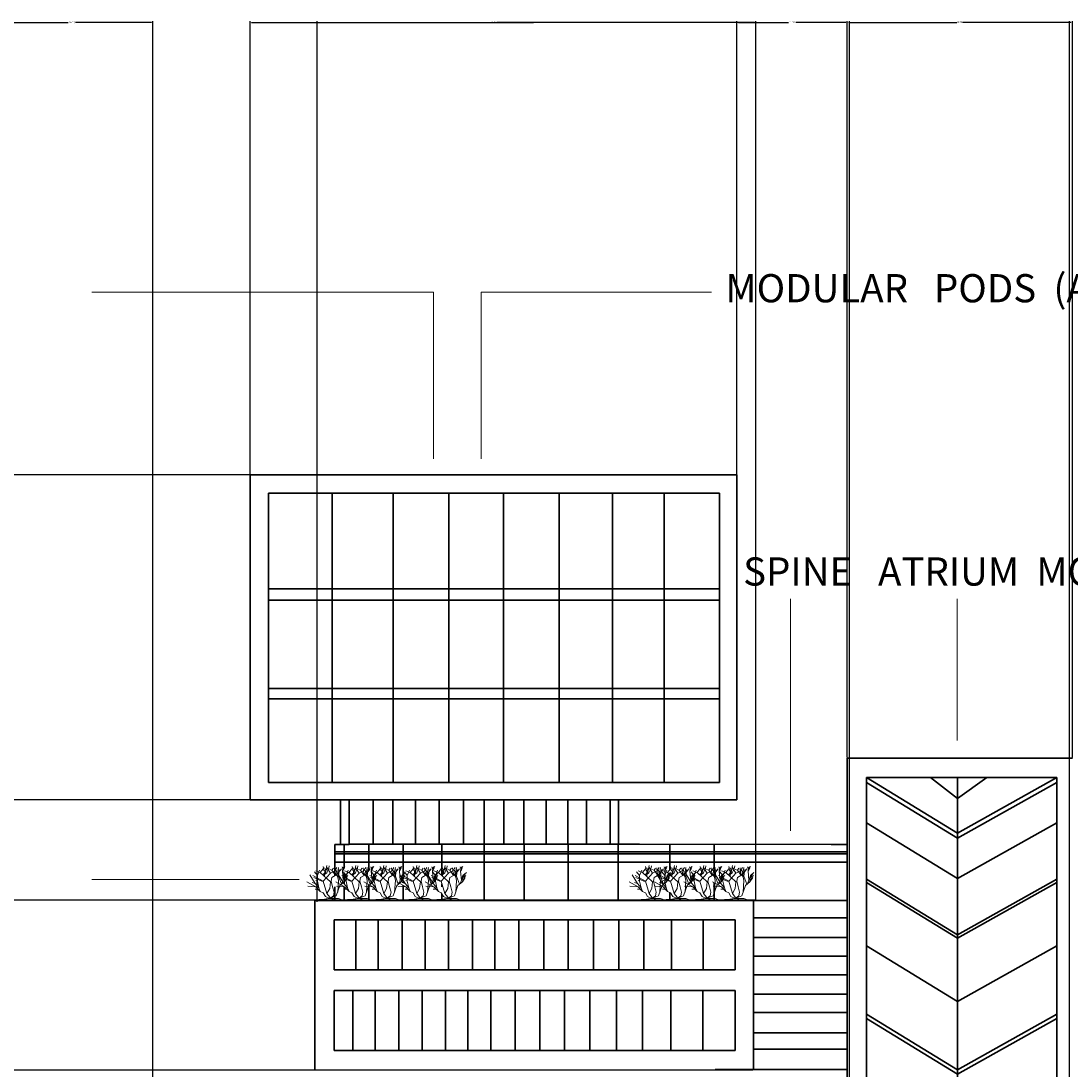
# Model space of a CAD drawing. Units: inches. Extents: x -160 to 434, y -145 to 103.
# Tile 3 of 7: x -26 to 107, y -31 to 103. Entities that reach past the tile are written whole.
import ezdxf

# ---------------------------------------------------------------- set-up
doc = ezdxf.new("R2010")
doc.units = ezdxf.units.IN
doc.header["$MEASUREMENT"] = 0
for name, color, linetype, lineweight in [('A-ANNO-DIMS', 2, 'Continuous', 18), ('A-ANNO-SYMB', 2, 'Continuous', 13), ('A-ANNO-TEXT', 3, 'Continuous', 18), ('A-ELEV', 7, 'Continuous', 35), ('L-PLNT', 3, 'Continuous', 13)]:
    doc.layers.add(name, color=color, linetype=linetype, lineweight=lineweight)
doc.styles.get("Standard").update_dxf_attribs({"font": 'arial.ttf'})
doc.dimstyles.get("Standard").update_dxf_attribs({"dimtxt": 0.18, "dimasz": 0.18, "dimexe": 0.18, "dimexo": 0.0625, "dimgap": 0.09, "dimtad": 0, "dimtih": 1, "dimtoh": 1, "dimdec": 4, "dimzin": 0, "dimdsep": 46, "dimtxsty": 'Standard', "dimcen": 0.09, "dimadec": 0, "dimazin": 0, "dimtfac": 1, "dimtdec": 4, "dimtofl": 0, "dimtmove": 0, "dimatfit": 3, "dimfxl": 1, "dimtolj": 1, "dimtzin": 0, "dimarcsym": 0})

# ---------------------------------------------------------------- blocks, each defined once
blk = doc.blocks.new('*U5')
for p, q in [((-12.471, 19.775), (-12.898, 22.044)), ((-11.28, 19.619), (-12.104, 21.184)), ((-11.433, 18.289), (-10.457, 22.749)), ((-8.16, 17.76), (-10.56, 21.6)), ((-9.48, 19.775), (-8.992, 22.592)), ((-7.2, 19.68), (-6.24, 21.12)), ((-5.086, 17.741), (-5.513, 21.34)), ((-5.28, 19.2), (-3.84, 21.6)), ((-3.377, 18.602), (-2.888, 21.575)), ((-0.508, 21.888), (-0.081, 20.558)), ((-0.203, 19.149), (0.102, 21.34)), ((-0.02, 20.01), (0.896, 21.105)), ((0.041, 20.714), (1.384, 22.044)), ((0.102, 21.34), (0.835, 21.888)), ((-18.24, 11.04), (-21.755, 16.655)), ((-12.96, 12.48), (-19.68, 16.32)), ((-13.92, 12.48), (-19.2, 14.88)), ((-16.8, 16.32), (-18.72, 18.72)), ((-14.88, 18.24), (-17.76, 19.2)), ((-16.8, 16.32), (-15.36, 19.68)), ((-16.8, 12.48), (-16.8, 16.32)), ((-14.88, 18.24), (-12.96, 20.64)), ((-8.16, 12), (-14.88, 18.24)), ((-13.325, 16.724), (-11.433, 18.289)), ((-12.96, 12.48), (-8.16, 17.76)), ((-11.677, 19.071), (-12.471, 19.775)), ((-12.043, 15.628), (-11.921, 18.836)), ((-11.982, 16.802), (-10.579, 18.054)), ((-11.921, 18.836), (-10.64, 20.401)), ((-10.579, 18.054), (-9.846, 19.697)), ((-7.2, 19.68), (-8.64, 20.16)), ((-8.16, 17.76), (-5.28, 19.2)), ((-7.68, 12.48), (-7.2, 14.88)), ((-4.8, 16.32), (-7.2, 19.68)), ((-7.2, 14.88), (-3.84, 16.8)), ((-3.377, 15.315), (-5.086, 17.819)), ((-2.88, 12.96), (-4.32, 19.68)), ((-3.84, 16.8), (-0.96, 20.64)), ((-2.766, 16.802), (-3.377, 18.602)), ((-2.88, 15.84), (-2.4, 20.16)), ((-0.96, 10.56), (-2.88, 15.84)), ((0.346, 13.203), (-0.203, 19.149)), ((-0.142, 19.384), (0.59, 20.401)), ((0.346, 13.203), (1.323, 16.254)), ((0.96, 12), (1.44, 15.36)), ((0.96, 12), (2.88, 14.88)), ((1.323, 16.254), (3.642, 18.289)), ((1.44, 15.36), (2.88, 17.28)), ((1.92, 13.44), (2.4, 15.36)), ((2.4, 15.36), (3.36, 16.32)), ((-17.76, 8.64), (-23.663, 11.961)), ((-17.76, 8.64), (-23.128, 9.222)), ((-18.24, 11.04), (-20.16, 11.52)), ((-15.84, 8.16), (-18.24, 11.04)), ((-16.32, 7.2), (-18.24, 7.2)), ((-16.8, 12.48), (-17.76, 12.96)), ((-14.88, 5.76), (-17.76, 8.64)), ((-15.84, 8.16), (-16.8, 12.48)), ((-14.88, 5.76), (-15.84, 8.16)), ((-12.96, 12.48), (-13.92, 12.48)), ((-10.56, 4.32), (-12.96, 12.48)), ((-10.56, 4.32), (-8.64, 7.68)), ((-8.64, 7.68), (-8.16, 12)), ((-6.72, 8.64), (-7.68, 12.48)), ((-5.76, 5.28), (-6.72, 8.64)), ((-4.32, 2.88), (-1.92, 9.6)), ((-3.36, 5.28), (-2.88, 12.96)), ((-1.92, 9.6), (0.96, 12)), ((-0.48, 10.8), (0.346, 13.203)), ((-15.84, 0.48), (-17.76, 0)), ((-13.44, 0.48), (-15.84, 0.48)), ((-12.96, 4.8), (-14.88, 5.76)), ((-9.6, 0.96), (-13.44, 0.48)), ((-11.52, 2.4), (-12.96, 4.8)), ((-9.6, 0.96), (-12.96, 0)), ((-8.64, 0.96), (-11.52, 2.4)), ((-8.64, 1.92), (-10.56, 4.32)), ((-9.6, 0.96), (-7.68, 0.96)), ((-8.64, 0.96), (-4.32, 2.88)), ((-8.64, 0.96), (-6.24, 2.88)), ((-8.64, 0.96), (-8.64, 1.92)), ((-8.64, 0.96), (-2.88, 0.96)), ((-7.68, 0.96), (-6.24, 0.48)), ((-6.24, 2.88), (-5.76, 5.28)), ((-6.24, 0.48), (-3.36, 0)), ((-2.88, 0.96), (0, 0))]:
    blk.add_line(p, q)
blk = doc.blocks.new('*D15')
at = {"layer": 'A-ANNO-DIMS', "color": 0, "lineweight": -2, "transparency": 16777216}
for p, q in [((2.83, 44.89), (-114.3, 44.89)), ((-114.12, 44.71), (-114.12, -28.36)), ((-114.12, -101.79), (-114.12, -28.72)), ((-29.6, -101.97), (-114.3, -101.97))]:
    blk.add_line(p, q, dxfattribs=at)
at = {"layer": 'A-ANNO-DIMS', "color": 0, "transparency": 16777216}
for points in [[(-114.15, 44.71), (-114.09, 44.71), (-114.12, 44.89)], [(-114.15, -101.79), (-114.09, -101.79), (-114.12, -101.97)]]:
    blk.add_solid(points, dxfattribs=at)
at = {"layer": 'Defpoints', "color": 0, "transparency": 16777216}
for p in [(-114.12, 44.89), (2.89, 44.89), (-29.54, -101.97)]:
    blk.add_point(p, dxfattribs=at)
at = {"layer": 'A-ANNO-DIMS', "color": 0, "transparency": 16777216, "insert": (-114.12, -28.54), "char_height": 0.18, "attachment_point": 5}
blk.add_mtext('\\A1;146.87', dxfattribs=at)
blk = doc.blocks.new('*D24')
at = {"layer": 'A-ANNO-DIMS', "color": 0, "lineweight": -2, "transparency": 16777216}
for p, q in [((78.96, -81.39), (78.96, 102.5)), ((79.14, 102.32), (92.54, 102.32)), ((106.73, 102.32), (93.33, 102.32)), ((106.91, -81.39), (106.91, 102.5))]:
    blk.add_line(p, q, dxfattribs=at)
at = {"layer": 'A-ANNO-DIMS', "color": 0, "transparency": 16777216}
for points in [[(79.14, 102.35), (79.14, 102.29), (78.96, 102.32)], [(106.73, 102.35), (106.73, 102.29), (106.91, 102.32)]]:
    blk.add_solid(points, dxfattribs=at)
at = {"layer": 'Defpoints', "color": 0, "transparency": 16777216}
for p in [(106.91, 102.32), (78.96, -81.45), (106.91, -81.45)]:
    blk.add_point(p, dxfattribs=at)
at = {"layer": 'A-ANNO-DIMS', "color": 0, "transparency": 16777216, "insert": (92.94, 102.32), "char_height": 0.18, "attachment_point": 5}
blk.add_mtext('\\A1;27.95', dxfattribs=at)
blk = doc.blocks.new('*D26')
at = {"layer": 'A-ANNO-DIMS', "color": 0, "lineweight": -2, "transparency": 16777216}
for p, q in [((2.89, 44.96), (2.89, 102.5)), ((3.07, 102.32), (33.39, 102.32)), ((64.5, 102.32), (34.18, 102.32)), ((64.68, 44.96), (64.68, 102.5))]:
    blk.add_line(p, q, dxfattribs=at)
at = {"layer": 'A-ANNO-DIMS', "color": 0, "transparency": 16777216}
for points in [[(3.07, 102.35), (3.07, 102.29), (2.89, 102.32)], [(64.5, 102.35), (64.5, 102.29), (64.68, 102.32)]]:
    blk.add_solid(points, dxfattribs=at)
at = {"layer": 'Defpoints', "color": 0, "transparency": 16777216}
for p in [(64.68, 102.32), (2.89, 44.89), (64.68, 44.89)]:
    blk.add_point(p, dxfattribs=at)
at = {"layer": 'A-ANNO-DIMS', "color": 0, "transparency": 16777216, "insert": (33.79, 102.32), "char_height": 0.18, "attachment_point": 5}
blk.add_mtext('\\A1;61.78', dxfattribs=at)
blk = doc.blocks.new('*D27')
at = {"layer": 'A-ANNO-DIMS', "color": 0, "lineweight": -2, "transparency": 16777216}
for p, q in [((64.68, 44.96), (64.68, 102.5)), ((64.86, 102.32), (71.23, 102.32)), ((78.51, 102.32), (72.14, 102.32)), ((78.69, 9.01), (78.69, 102.5))]:
    blk.add_line(p, q, dxfattribs=at)
at = {"layer": 'A-ANNO-DIMS', "color": 0, "transparency": 16777216}
for points in [[(64.86, 102.35), (64.86, 102.29), (64.68, 102.32)], [(78.51, 102.35), (78.51, 102.29), (78.69, 102.32)]]:
    blk.add_solid(points, dxfattribs=at)
at = {"layer": 'Defpoints', "color": 0, "transparency": 16777216}
for p in [(78.69, 102.32), (64.68, 44.89), (78.69, 8.95)]:
    blk.add_point(p, dxfattribs=at)
at = {"layer": 'A-ANNO-DIMS', "color": 0, "transparency": 16777216, "insert": (71.68, 102.32), "char_height": 0.18, "attachment_point": 5}
blk.add_mtext('\\A1;14.013', dxfattribs=at)
blk = doc.blocks.new('*D28')
at = {"layer": 'A-ANNO-DIMS', "color": 0, "lineweight": -2, "transparency": 16777216}
for p, q in [((78.69, 9.01), (78.69, 102.5)), ((78.87, 102.32), (92.58, 102.32)), ((107.09, 102.32), (93.38, 102.32)), ((107.27, 9.01), (107.27, 102.5))]:
    blk.add_line(p, q, dxfattribs=at)
at = {"layer": 'A-ANNO-DIMS', "color": 0, "transparency": 16777216}
for points in [[(78.87, 102.35), (78.87, 102.29), (78.69, 102.32)], [(107.09, 102.35), (107.09, 102.29), (107.27, 102.32)]]:
    blk.add_solid(points, dxfattribs=at)
at = {"layer": 'Defpoints', "color": 0, "transparency": 16777216}
for p in [(107.27, 102.32), (78.69, 8.95), (107.27, 8.95)]:
    blk.add_point(p, dxfattribs=at)
at = {"layer": 'A-ANNO-DIMS', "color": 0, "transparency": 16777216, "insert": (92.98, 102.32), "char_height": 0.18, "attachment_point": 5}
blk.add_mtext('\\A1;28.58', dxfattribs=at)
blk = doc.blocks.new('*D29')
at = {"layer": 'A-ANNO-DIMS', "color": 0, "lineweight": -2, "transparency": 16777216}
for p, q in [((2.83, 44.89), (-114.3, 44.89)), ((-114.12, 44.71), (-114.12, 24.46)), ((-114.12, 3.84), (-114.12, 24.1)), ((2.83, 3.66), (-114.3, 3.66))]:
    blk.add_line(p, q, dxfattribs=at)
at = {"layer": 'A-ANNO-DIMS', "color": 0, "transparency": 16777216}
for points in [[(-114.15, 44.71), (-114.09, 44.71), (-114.12, 44.89)], [(-114.15, 3.84), (-114.09, 3.84), (-114.12, 3.66)]]:
    blk.add_solid(points, dxfattribs=at)
at = {"layer": 'Defpoints', "color": 0, "transparency": 16777216}
for p in [(2.89, 44.89), (-114.12, 3.66), (2.89, 3.66)]:
    blk.add_point(p, dxfattribs=at)
at = {"layer": 'A-ANNO-DIMS', "color": 0, "transparency": 16777216, "insert": (-114.12, 24.28), "char_height": 0.18, "attachment_point": 5}
blk.add_mtext('\\A1;41.23', dxfattribs=at)
blk = doc.blocks.new('*D30')
at = {"layer": 'A-ANNO-DIMS', "color": 0, "lineweight": -2, "transparency": 16777216}
for p, q in [((2.83, 3.66), (-114.3, 3.66)), ((-114.12, 3.48), (-114.12, -32.35)), ((-114.12, -68.55), (-114.12, -32.72)), ((-9.37, -68.73), (-114.3, -68.73))]:
    blk.add_line(p, q, dxfattribs=at)
at = {"layer": 'A-ANNO-DIMS', "color": 0, "transparency": 16777216}
for points in [[(-114.15, 3.48), (-114.09, 3.48), (-114.12, 3.66)], [(-114.15, -68.55), (-114.09, -68.55), (-114.12, -68.73)]]:
    blk.add_solid(points, dxfattribs=at)
at = {"layer": 'Defpoints', "color": 0, "transparency": 16777216}
for p in [(-114.12, 3.66), (2.89, 3.66), (-9.31, -68.73)]:
    blk.add_point(p, dxfattribs=at)
at = {"layer": 'A-ANNO-DIMS', "color": 0, "transparency": 16777216, "insert": (-114.12, -32.54), "char_height": 0.18, "attachment_point": 5}
blk.add_mtext('\\A1;72.4', dxfattribs=at)
blk = doc.blocks.new('*D33')
at = {"layer": 'A-ANNO-DIMS', "color": 0, "lineweight": -2, "transparency": 16777216}
for p, q in [((11.38, -9.29), (11.38, 102.5)), ((11.56, 102.32), (38.86, 102.32)), ((66.91, 102.32), (39.62, 102.32)), ((67.09, -9.01), (67.09, 102.5))]:
    blk.add_line(p, q, dxfattribs=at)
at = {"layer": 'A-ANNO-DIMS', "color": 0, "transparency": 16777216}
for points in [[(11.56, 102.35), (11.56, 102.29), (11.38, 102.32)], [(66.91, 102.35), (66.91, 102.29), (67.09, 102.32)]]:
    blk.add_solid(points, dxfattribs=at)
at = {"layer": 'Defpoints', "color": 0, "transparency": 16777216}
for p in [(67.09, 102.32), (67.09, -9.07), (11.38, -9.35)]:
    blk.add_point(p, dxfattribs=at)
at = {"layer": 'A-ANNO-DIMS', "color": 0, "transparency": 16777216, "insert": (39.24, 102.32), "char_height": 0.18, "attachment_point": 5}
blk.add_mtext('\\A1;55.71', dxfattribs=at)
blk = doc.blocks.new('*D34')
at = {"layer": 'A-ANNO-DIMS', "color": 0, "lineweight": -2, "transparency": 16777216}
for p, q in [((67.03, -9.07), (-114.3, -9.07)), ((-114.12, -9.25), (-114.12, -19.67)), ((-114.12, -30.46), (-114.12, -20.04)), ((66.72, -30.64), (-114.3, -30.64))]:
    blk.add_line(p, q, dxfattribs=at)
at = {"layer": 'A-ANNO-DIMS', "color": 0, "transparency": 16777216}
for points in [[(-114.15, -9.25), (-114.09, -9.25), (-114.12, -9.07)], [(-114.15, -30.46), (-114.09, -30.46), (-114.12, -30.64)]]:
    blk.add_solid(points, dxfattribs=at)
at = {"layer": 'Defpoints', "color": 0, "transparency": 16777216}
for p in [(67.09, -9.07), (-114.12, -30.64), (66.78, -30.64)]:
    blk.add_point(p, dxfattribs=at)
at = {"layer": 'A-ANNO-DIMS', "color": 0, "transparency": 16777216, "insert": (-114.12, -19.85), "char_height": 0.18, "attachment_point": 5}
blk.add_mtext('\\A1;21.567', dxfattribs=at)
blk = doc.blocks.new('*D47')
at = {"layer": 'A-ANNO-DIMS', "color": 0, "lineweight": -2, "transparency": 16777216}
for p, q in [((-30.07, -67.91), (-30.07, 102.5)), ((-29.89, 102.32), (-20.23, 102.32)), ((-9.63, 102.32), (-19.3, 102.32)), ((-9.45, -53.37), (-9.45, 102.5))]:
    blk.add_line(p, q, dxfattribs=at)
at = {"layer": 'A-ANNO-DIMS', "color": 0, "transparency": 16777216}
for points in [[(-29.89, 102.35), (-29.89, 102.29), (-30.07, 102.32)], [(-9.63, 102.35), (-9.63, 102.29), (-9.45, 102.32)]]:
    blk.add_solid(points, dxfattribs=at)
at = {"layer": 'Defpoints', "color": 0, "transparency": 16777216}
for p in [(-9.45, 102.32), (-9.45, -53.43), (-30.07, -67.97)]:
    blk.add_point(p, dxfattribs=at)
at = {"layer": 'A-ANNO-DIMS', "color": 0, "transparency": 16777216, "insert": (-19.76, 102.32), "char_height": 0.18, "attachment_point": 5}
blk.add_mtext('\\A1;20.625', dxfattribs=at)

msp = doc.modelspace()

# ---------------------------------------------------------------- linework, layer by layer
at = {"layer": 'A-ANNO-SYMB'}
for p, q in [((26.1523, 68.0806), (-17.2202, 68.0806)), ((26.1523, 46.924), (26.1523, 68.0806)), ((32.2042, 46.924), (32.2042, 68.0806)), ((32.2042, 68.0806), (61.4554, 68.0806)), ((71.4813, -0.2968), (71.4813, 29.1663)), ((92.6493, 11.2011), (92.6493, 29.1663)), ((9.0899, -6.4717), (-17.2202, -6.4717))]:
    msp.add_line(p, q, dxfattribs=at)
at = {"layer": 'A-ELEV'}
for p, q in [((2.8933, 44.8926), (64.6783, 44.8926)), ((2.8933, 3.6646), (2.8933, 44.8926)), ((64.6783, 44.8926), (64.6783, 3.6646)), ((5.2218, 42.5669), (62.4791, 42.5669)), ((5.2218, 5.8612), (5.2218, 42.5669)), ((13.2971, 5.8612), (13.2971, 42.5669)), ((21.0273, 5.8612), (21.0273, 42.5669)), ((28.0963, 5.8612), (28.0963, 42.5669)), ((35.0319, 5.8612), (35.0319, 42.5669)), ((42.1009, 5.8612), (42.1009, 42.5669)), ((48.9032, 5.8612), (48.9032, 42.5669)), ((55.4387, 5.8612), (55.4387, 42.5669)), ((62.4791, 42.5669), (62.4791, 5.8612)), ((5.2218, 30.444), (62.4791, 30.444)), ((5.2218, 28.9786), (62.4791, 28.9786)), ((5.2218, 17.7883), (62.4791, 17.7883)), ((5.2218, 16.4562), (62.4791, 16.4562)), ((78.691, -2.0014), (78.691, 8.9457)), ((78.691, 8.9457), (107.2684, 8.9457)), ((62.4791, 5.8612), (5.2218, 5.8612)), ((81.1405, -2.0014), (81.1405, 6.4991)), ((81.1405, 6.4991), (105.2782, 6.4991)), ((81.1405, 6.4991), (92.6738, -0.5657)), ((81.1405, 5.8372), (92.6738, -1.2276)), ((92.6738, 3.8393), (89.2731, 6.4991)), ((92.6738, -2.0014), (92.6738, 6.4991)), ((105.2782, 6.4991), (92.6738, -0.5657)), ((92.6738, 3.8393), (96.4036, 6.4991)), ((105.2782, 5.8372), (92.6738, -1.2276)), ((105.2782, 6.4991), (105.2782, -38.311)), ((64.6783, 3.6646), (2.8933, 3.6646)), ((14.341, 3.6652), (14.341, -1.996)), ((15.4432, 3.6652), (15.4432, -1.996)), ((18.518, 3.6652), (18.518, -1.996)), ((21.0086, 3.6652), (21.0086, -1.996)), ((23.8824, 3.6652), (23.8824, -1.996)), ((26.8839, 3.6652), (26.8839, -1.996)), ((29.9492, 3.6652), (29.9492, -1.996)), ((32.5985, 3.6652), (32.5985, -1.996)), ((35.0712, 3.6652), (35.0712, -1.996)), ((37.6322, 3.6652), (37.6322, -1.996)), ((40.4581, 3.6652), (40.4581, -1.996)), ((43.1957, 3.6652), (43.1957, -1.996)), ((45.5801, 3.6652), (45.5801, -1.996)), ((48.5891, -1.996), (48.5891, 3.6652)), ((49.6267, -1.996), (49.6267, 3.6652)), ((81.1405, 0.7458), (92.6738, -6.319)), ((105.2782, 0.7458), (92.6738, -6.319)), ((13.6521, -2.0014), (14.341, -1.996)), ((13.6521, -2.0014), (13.6521, -5.9856)), ((14.8156, -2.0014), (13.6521, -2.0014)), ((14.8156, -2.0014), (14.8156, -5.0152)), ((14.8156, -2.0014), (15.4432, -2.0014)), ((29.896, -1.996), (15.4432, -1.996)), ((17.9418, -2.0014), (17.9418, -5.3313)), ((22.3267, -2.0014), (22.3267, -5.9609)), ((27.2394, -2.0014), (27.2394, -5.7186)), ((29.896, -1.996), (51.2734, -1.996)), ((32.5987, -2.0014), (32.5987, -7.382)), ((37.6729, -2.0014), (37.6729, -7.382)), ((43.2421, -2.0014), (43.2421, -7.382)), ((49.6159, -2.0014), (49.6159, -7.382)), ((52.3111, -1.996), (51.2734, -1.996)), ((52.3111, -1.996), (78.691, -2.0036)), ((56.1752, -2.0014), (56.1752, -5.2019)), ((61.8064, -2.0014), (61.8064, -6.093)), ((76.6235, -2.0014), (78.691, -2.0014)), ((78.691, -2.0014), (78.691, -56.1669)), ((81.1405, -2.0014), (81.1405, -53.5674)), ((92.6738, -2.0014), (92.6738, -53.5674)), ((13.6521, -2.938), (14.341, -2.9327)), ((13.6521, -3.2112), (14.341, -3.2059)), ((29.896, -2.9327), (14.341, -2.9327)), ((29.896, -3.2059), (14.341, -3.2059)), ((29.896, -2.9327), (51.2734, -2.9327)), ((29.896, -3.2059), (51.2734, -3.2059)), ((52.3111, -2.9327), (51.2734, -2.9327)), ((52.3111, -3.2059), (51.2734, -3.2059)), ((52.3111, -2.9327), (78.691, -2.9403)), ((52.3111, -3.2059), (78.691, -3.2135)), ((13.6521, -4.265), (14.341, -4.2597)), ((29.896, -4.2597), (14.341, -4.2597)), ((29.896, -4.2597), (51.2734, -4.2597)), ((52.3111, -4.2597), (51.2734, -4.2597)), ((52.3111, -4.2597), (78.691, -4.2673)), ((14.8156, -5.6171), (14.8156, -6.3043)), ((22.3267, -6.1608), (22.3267, -6.364)), ((22.3267, -6.5861), (22.3267, -6.8911)), ((56.1752, -5.6217), (56.1752, -5.9558)), ((56.1752, -6.6245), (56.1752, -6.6707)), ((81.1405, -6.3991), (92.6738, -13.4639)), ((105.2782, -6.3991), (92.6738, -13.4639)), ((13.6521, -7.382), (13.6521, -9.1182)), ((14.8156, -6.7758), (14.8156, -6.9778)), ((14.8156, -7.3715), (14.8156, -7.382)), ((14.8156, -7.382), (14.8156, -9.1182)), ((17.9418, -7.118), (17.9418, -7.382)), ((17.9418, -7.382), (17.9418, -9.1182)), ((22.3267, -7.2301), (22.3267, -7.382)), ((22.3267, -7.382), (22.3267, -9.1182)), ((27.2394, -6.9897), (27.2394, -7.382)), ((32.5987, -7.382), (32.5987, -9.1182)), ((37.6729, -7.382), (37.6729, -9.1182)), ((43.2421, -7.382), (43.2421, -9.1182)), ((49.6159, -7.382), (49.6159, -9.1182)), ((61.8064, -6.8984), (61.8064, -7.382)), ((61.8064, -7.382), (61.8064, -9.1182)), ((81.1405, -6.8573), (92.6738, -13.9221)), ((105.2782, -6.8573), (92.6738, -13.9221)), ((25.4205, -9.1182), (11.0861, -9.1182)), ((11.0861, -9.1182), (11.0861, -30.6379)), ((25.4205, -9.1182), (61.9316, -9.1182)), ((27.2394, -8.3044), (27.2394, -9.1182)), ((56.1752, -8.1076), (56.1752, -9.1182)), ((61.8064, -9.1182), (78.691, -9.1182)), ((66.7815, -9.1182), (66.7815, -24.7325)), ((25.8596, -11.5815), (13.529, -11.5815)), ((13.529, -11.5815), (13.529, -17.9165)), ((16.3153, -11.5815), (16.3153, -17.9165)), ((19.1377, -11.5815), (19.1377, -17.9165)), ((22.1617, -11.5815), (22.1617, -17.9165)), ((25.1184, -11.5815), (25.1184, -17.9165)), ((25.8596, -11.5815), (60.4046, -11.5815)), ((28.0752, -11.5815), (28.0752, -17.9165)), ((31.0998, -11.5815), (31.0998, -17.9165)), ((33.9331, -11.5815), (33.9331, -17.9165)), ((36.996, -11.5815), (36.996, -17.9165)), ((40.1738, -11.5815), (40.1738, -17.9165)), ((43.2751, -11.5815), (43.2751, -17.9165)), ((46.4912, -11.5815), (46.4912, -17.9165)), ((49.669, -11.5815), (49.669, -17.9165)), ((52.8468, -11.5815), (52.8468, -17.9165)), ((56.3794, -11.5815), (56.3794, -17.9165)), ((60.4046, -11.5815), (60.4046, -17.9165)), ((60.4046, -11.5815), (64.4675, -11.5815)), ((64.4675, -11.5815), (64.4675, -17.9165)), ((66.7815, -11.3428), (78.691, -11.3428)), ((66.7815, -13.813), (78.691, -13.813)), ((81.1405, -14.8673), (92.6738, -21.9321)), ((105.2782, -14.8673), (92.6738, -21.9321)), ((66.7815, -16.1938), (78.691, -16.1938)), ((60.4046, -17.9165), (13.529, -17.9165)), ((64.4675, -17.9165), (60.4046, -17.9165)), ((66.7815, -18.5527), (78.691, -18.5527)), ((60.3669, -20.5338), (13.529, -20.5338)), ((13.529, -20.5338), (13.529, -28.1746)), ((13.529, -20.5338), (13.529, -24.1167)), ((15.9283, -20.5338), (15.9283, -28.1746)), ((18.7507, -20.5338), (18.7507, -28.1746)), ((21.7746, -20.5338), (21.7746, -28.1746)), ((24.7314, -20.5338), (24.7314, -28.1746)), ((27.6881, -20.5338), (27.6881, -28.1746)), ((30.5108, -20.5338), (30.5108, -28.1746)), ((33.4308, -20.5338), (33.4308, -28.1746)), ((36.5454, -20.5338), (36.5454, -28.1746)), ((39.6601, -20.5338), (39.6601, -28.1746)), ((42.7747, -20.5338), (42.7747, -28.1746)), ((45.9867, -20.5338), (45.9867, -28.1746)), ((49.3934, -20.5338), (49.3934, -28.1746)), ((52.7027, -20.5338), (52.7027, -28.1746)), ((56.304, -20.5338), (56.304, -28.1746)), ((60.3669, -28.1746), (60.3669, -20.5338)), ((60.3669, -20.5338), (64.4675, -20.5338)), ((64.4675, -20.5338), (64.4675, -21.2493)), ((64.4675, -21.2493), (64.4675, -27.5844)), ((66.7815, -21.0198), (78.691, -21.0198)), ((66.7815, -23.3426), (78.691, -23.3426)), ((81.1405, -23.5428), (92.6738, -30.6076)), ((105.2782, -23.5428), (92.6738, -30.6076)), ((66.7815, -30.6379), (66.7815, -24.7325)), ((81.1405, -24.1029), (92.6738, -31.1677)), ((105.2782, -24.1029), (92.6738, -31.1677)), ((66.7815, -25.9263), (78.691, -25.9263)), ((64.4675, -27.5844), (64.4675, -27.5844)), ((64.4675, -28.1746), (64.4675, -27.5844)), ((13.529, -28.1746), (60.3669, -28.1746)), ((60.3669, -28.1746), (64.4675, -28.1746)), ((66.7815, -27.9932), (78.691, -27.9932)), ((61.9316, -30.5875), (78.691, -30.5875))]:
    msp.add_line(p, q, dxfattribs=at)

# ---------------------------------------------------------------- block references
at = {"layer": 'L-PLNT', "xscale": 0.1923638725067976, "yscale": 0.1923638725067976, "zscale": 0.1923638725067976}
for p in [(14.6463, -9.0714), (18.2992, -9.0714), (21.8761, -9.0714), (26.0617, -9.0714), (29.6386, -9.0714), (55.5526, -9.0714), (58.749, -9.0714), (62.478, -9.0714), (66.131, -9.0714)]:
    msp.add_blockref('*U5', p, dxfattribs=at)

# ---------------------------------------------------------------- texts
at = {"layer": 'A-ANNO-TEXT'}
for s, p in [('MODULAR   PODS  (A , B , ATRIUM)', (63.2171, 66.798)), ('SPINE   ATRIUM  MODULE', (65.4677, 30.8438))]:
    msp.add_text(s, height=3.579169, dxfattribs=at).set_placement(p)

# ---------------------------------------------------------------- dimensions: what is measured, and where the dimension line sits
at = {"layer": 'A-ANNO-DIMS'}
for base, p1, p2, override, picture, middle in [((-9.4492, 102.3218), (-30.0745, -67.9742), (-9.4492, -53.4308), {"dimdec": 3, "dimlfac": 1, "dimrnd": 0, "dimzin": 0, "dimdsep": 46, "dimlunit": 2}, '*D47', (-19.7619, 102.3218)), ((64.67825, 102.32183), (2.8933, 44.89259), (64.67825, 44.89259), {"dimdec": 2, "dimlfac": 1, "dimrnd": 0, "dimzin": 0, "dimdsep": 46, "dimlunit": 2}, '*D26', (33.78578, 102.32183)), ((67.0945, 102.3218), (11.383, -9.3536), (67.0945, -9.0714), {"dimdec": 2, "dimlfac": 1, "dimrnd": 0, "dimzin": 0, "dimdsep": 46, "dimlunit": 2}, '*D33', (39.2387, 102.3218)), ((78.691, 102.3218), (64.6783, 44.8926), (78.691, 8.9457), {"dimdec": 3, "dimlfac": 1, "dimrnd": 0, "dimzin": 0, "dimdsep": 46, "dimlunit": 2}, '*D27', (71.6846, 102.3218)), ((107.2684, 102.3218), (78.691, 8.9457), (107.2684, 8.9457), {"dimdec": 2, "dimlfac": 1, "dimrnd": 0, "dimzin": 0, "dimdsep": 46, "dimlunit": 2}, '*D28', (92.9797, 102.3218)), ((106.9124, 102.3218), (78.9633, -81.4546), (106.9124, -81.4546), {"dimdec": 2, "dimlfac": 1, "dimrnd": 0, "dimzin": 0, "dimdsep": 46, "dimlunit": 2}, '*D24', (92.9378, 102.3218))]:
    dim = msp.add_linear_dim(base=base, p1=p1, p2=p2, dimstyle='Standard', override=override, dxfattribs=at)
    dim.commit()
    dim.dimension.update_dxf_attribs({"geometry": picture, "text_midpoint": middle})
for base, p1, p2, override, picture, middle in [((-114.1222, 44.8926), (-29.5407, -101.9747), (2.8933, 44.8926), {"dimdec": 2, "dimlfac": 1, "dimrnd": 0, "dimzin": 0, "dimdsep": 46, "dimlunit": 2}, '*D15', (-114.1222, -28.5411)), ((-114.1222, 3.6646), (2.8933, 44.8926), (2.8933, 3.6646), {"dimdec": 2, "dimlfac": 1, "dimrnd": 0, "dimzin": 0, "dimdsep": 46, "dimlunit": 2}, '*D29', (-114.1222, 24.2786)), ((-114.1222, 3.6646), (-9.3089, -68.735), (2.8933, 3.6646), {"dimdec": 1, "dimlfac": 1, "dimrnd": 0, "dimzin": 0, "dimdsep": 46, "dimlunit": 2}, '*D30', (-114.1222, -32.5352)), ((-114.12224, -30.63792), (67.09448, -9.07136), (66.78146, -30.63791), {"dimdec": 3, "dimlfac": 1, "dimrnd": 0, "dimzin": 0, "dimdsep": 46, "dimlunit": 2}, '*D34', (-114.12224, -19.85463))]:
    dim = msp.add_linear_dim(base=base, p1=p1, p2=p2, angle=90, dimstyle='Standard', override=override, dxfattribs=at)
    dim.commit()
    dim.dimension.update_dxf_attribs({"geometry": picture, "text_midpoint": middle})

doc.saveas('drawing.dxf')
